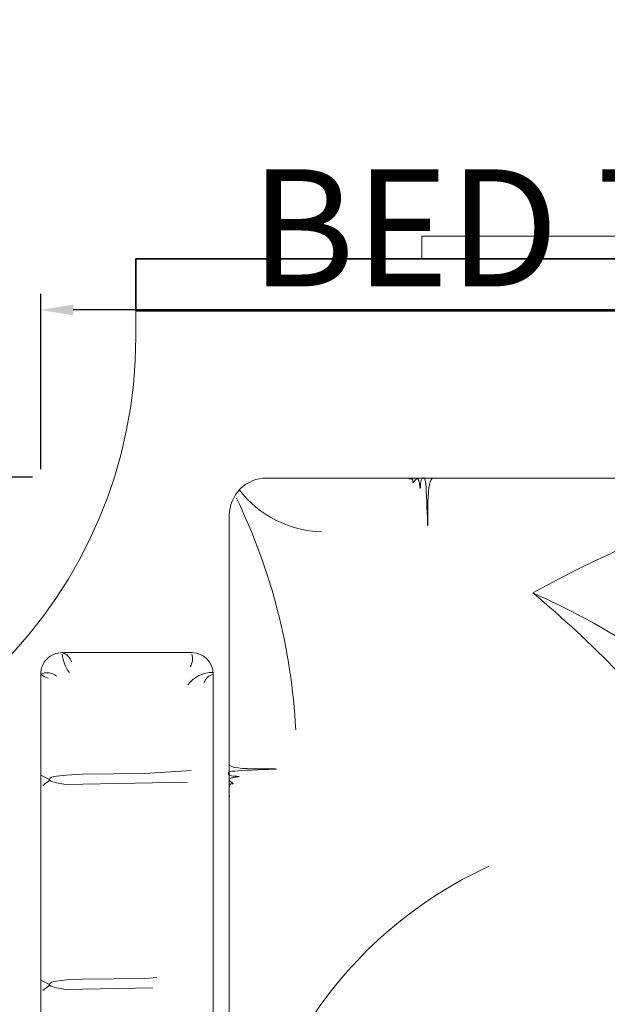
# Model space of a CAD drawing. Units: inches. Extents: x 3321 to 5237, y 11 to 1752.
# Tile 17 of 43: x 4367 to 4413, y 1230 to 1306. Entities that reach past the tile are written whole.
import ezdxf

# ---------------------------------------------------------------- set-up
doc = ezdxf.new("R2010")
doc.units = ezdxf.units.IN
for name, color, linetype, lineweight in [('A-ANNO-DIMS', 2, 'Continuous', 18), ('A-DOOR', 4, 'Continuous', 18), ('A-WALL', 7, 'Continuous', 35), ('FUR', 42, 'Continuous', 18)]:
    doc.layers.add(name, color=color, linetype=linetype, lineweight=lineweight)
doc.styles.get("Standard").update_dxf_attribs({"font": 'arial.ttf'})
doc.dimstyles.new('ISO-25', dxfattribs={"dimtxt": 9, "dimasz": 2.5, "dimexe": 1.25, "dimexo": 0.625, "dimtad": 1, "dimdec": 1, "dimlunit": 3, "dimtxsty": 'Standard', "dimcen": 2.5, "dimclrd": 4, "dimclre": 4, "dimclrt": 256, "dimadec": 0, "dimazin": 0, "dimtfac": 1, "dimtdec": 1, "dimtmove": 0, "dimatfit": 3, "dimfxl": 1, "dimarcsym": 0})

# ---------------------------------------------------------------- blocks, each defined once
blk = doc.blocks.new('*U9')
for p, q in [((-36, 0), (-36, 6)), ((0, 0), (0, 6))]:
    blk.add_line(p, q)
blk.add_lwpolyline([(0, 0), (0, -36), (-1.75, -36), (-1.75, 0)], close=True)
blk.add_arc((0, 0), 36, 180, 270)
blk = doc.blocks.new('*U5')
for p, q in [((0, 0), (0, -6)), ((-30, 0), (-30, -6))]:
    blk.add_line(p, q)
blk.add_lwpolyline([(0, 0), (0, 30), (-1.75, 30), (-1.75, 0)], close=True)
blk.add_arc((0, 0), 30, 90, 180)
blk = doc.blocks.new('*X127')
at = {"color": 0}
for p, q in [((3155.9, 8182.9), (3155.9, 8182.9)), ((3147.8, 8143.4), (3147.8, 8143.4)), ((3283, 8049.6), (3283, 8049.6)), ((3209.5, 8023.9), (3209.5, 8023.9)), ((3251.6, 7997), (3251.6, 7997)), ((3154.1, 7950.7), (3154.1, 7950.7))]:
    blk.add_line(p, q, dxfattribs=at)
blk = doc.blocks.new('*X126')
at = {"color": 0}
for p, q in [((3155.9, 8182.9), (3155.9, 8182.9)), ((3139.8, 7939.7), (3139.8, 7939.7))]:
    blk.add_line(p, q, dxfattribs=at)
blk = doc.blocks.new('*X125')
at = {"color": 0}
for p, q in [((3155.9, 8182.9), (3155.9, 8182.9)), ((3139.8, 7939.7), (3139.8, 7939.7))]:
    blk.add_line(p, q, dxfattribs=at)
blk = doc.blocks.new('*X124')
at = {"color": 0}
for p, q in [((3163, 7776.2), (3163, 7776.2)), ((3422.2, 7761.3), (3422.2, 7761.3)), ((3244.3, 7698.6), (3244.3, 7698.6)), ((3236.2, 7675.7), (3236.2, 7675.7)), ((3340.3, 7689.4), (3340.3, 7689.4))]:
    blk.add_line(p, q, dxfattribs=at)
blk = doc.blocks.new('BED1')
for p, q in [((0, -1000), (0, 800)), ((150, 800), (0, 800)), ((150, 800), (150, -1000)), ((2058.7, 800), (150, 800)), ((528, 800), (528, -1000)), ((211.8, 614.9), (277.5, 585.4)), ((2537.2, 404.9), (2237.2, 404.9)), ((2187.2, 354.9), (2187.2, -545.1)), ((2587.2, -545.1), (2587.2, 354.9)), ((2582, 188.1), (2565.4, 174.8)), ((2566.3, 178.5), (2565.2, 177.4)), ((2565.4, 174.8), (2585.7, 165.4)), ((2566.3, -296.8), (2565.2, -297.9)), ((2582, -287.1), (2565.4, -300.5)), ((2565.4, -300.5), (2585.7, -309.9)), ((2237.2, -595.1), (2537.2, -595.1)), ((150, -1000), (0, -1000)), ((150, -1000), (2063.5, -1000))]:
    blk.add_line(p, q)
for points in [[(934, 797.9), (930.9, 797.7), (928.3, 797.4), (926.3, 796.9), (924.9, 796.3), (923.8, 795.6), (923.1, 794.8), (922.7, 793.8), (922.5, 792.7), (922.4, 791.5), (922.5, 790.3), (922.6, 789.2), (922.6, 788.3), (922.6, 787.6), (922.4, 787.3), (922, 787.4), (921.4, 787.9), (920.6, 788.9), (919.5, 790.2), (918.4, 791.6), (917.1, 793.1), (915.9, 794.6), (914.6, 796), (913.3, 797.1), (912.2, 797.9), (911.1, 798.3), (910.1, 798.4), (909.2, 798), (908.3, 797.1), (907.5, 795.8), (906.8, 793.9), (906, 791.4), (905.4, 788.5), (904.8, 785.2), (904.2, 781.7), (903.7, 778.4), (903.2, 775.4), (902.8, 772.9), (902.5, 771.3), (902.3, 770.6), (902.1, 771.2), (902, 772.8), (901.8, 775.2), (901.7, 778.1), (901.5, 781.5), (901.2, 785), (900.8, 788.4), (900.2, 791.5), (899.5, 794.1), (898.6, 796.2), (897.6, 797.9), (896.5, 799.2), (895.3, 800), (894.1, 800.5), (893, 800.7), (891.9, 800.5), (890.9, 800.1), (890, 799), (889.1, 797.1), (888.3, 794), (887.6, 789.3), (886.9, 782.9), (886.2, 774.2), (885.5, 763.1), (884.8, 749.5), (884.2, 734.2), (883.6, 718.3), (883, 702.8), (882.5, 688.8), (882, 677.5), (881.7, 669.8), (881.5, 666.9), (881.3, 669.4), (881.3, 676.7), (881.3, 687.8), (881.2, 701.5), (881.1, 716.8), (880.8, 732.6), (880.2, 748), (879.4, 761.8), (878.3, 773.2), (876.9, 782.2), (875.1, 789.2), (872.9, 794.4), (870.3, 798), (869, 799)], [(2150, -913.5), (2150, 723.2)], [(2327.6, 182.3), (2530, 185.9), (2550.8, 181.9), (2561.7, 179), (2566, 176.7), (2566.9, 174.4), (2566.3, 171.9), (2562, 169.2), (2550.3, 166.5), (2527.7, 163.9), (2490.6, 161.8), (2345.5, 160.2), (2317.8, 158.5)], [(494.7, 3.1), (458.9, 95.3)], [(2149.7, -259.9), (2150, -268.4), (2150.1, -274.1), (2150.1, -278.1), (2150, -281.4), (2149.8, -284), (2149.5, -286.1), (2149.1, -287.8), (2148.7, -289), (2148.1, -289.9), (2147.4, -290.5), (2146.6, -290.8), (2145.6, -291), (2144.6, -291), (2143.6, -291), (2142.7, -290.9), (2141.9, -290.9), (2141.4, -290.9), (2141.1, -291), (2141.2, -291.4), (2141.7, -291.9), (2142.5, -292.6), (2143.5, -293.4), (2144.7, -294.4), (2146, -295.4), (2147.2, -296.5), (2148.4, -297.6), (2149.3, -298.6), (2150, -299.6), (2150.3, -300.5), (2150.4, -301.3), (2150, -302.1), (2149.3, -302.8), (2148.2, -303.5), (2146.6, -304.1), (2144.6, -304.7), (2142.1, -305.2), (2139.3, -305.7), (2136.5, -306.2), (2133.7, -306.6), (2131.2, -307), (2129.2, -307.3), (2127.8, -307.6), (2127.3, -307.8), (2127.7, -308), (2129, -308.1), (2131, -308.2), (2133.5, -308.3), (2136.3, -308.5), (2139.2, -308.7), (2142, -309), (2144.6, -309.5), (2146.8, -310.1), (2148.6, -310.9), (2150, -311.7), (2151, -312.7), (2151.7, -313.6), (2152.1, -314.6), (2152.3, -315.6), (2152.2, -316.5), (2151.8, -317.3), (2150.9, -318.1), (2149.3, -318.8), (2146.7, -319.4), (2142.8, -320), (2137.4, -320.6), (2130.2, -321.2), (2121, -321.8), (2109.7, -322.3), (2096.9, -322.9), (2083.6, -323.4), (2070.7, -323.9), (2059.1, -324.3), (2049.6, -324.7), (2043.2, -325), (2040.8, -325.2), (2042.9, -325.3), (2049, -325.3), (2058.2, -325.3), (2069.6, -325.4), (2082.3, -325.5), (2095.6, -325.8), (2108.4, -326.2), (2119.9, -326.8), (2129.4, -327.8), (2136.9, -329), (2142.7, -330.5), (2147, -332.3), (2150, -334.4), (2150.9, -335.6)], [(2246.5, -294.4), (2530, -289.4), (2550.8, -293.4), (2561.7, -296.3), (2566, -298.6), (2566.9, -300.8), (2566.3, -303.4), (2562, -306.1), (2550.3, -308.8), (2527.7, -311.3), (2490.6, -313.5), (2345.5, -315), (2238.6, -321.8)], [(1733.7, -998.3), (1731.1, -998.1), (1729, -997.8), (1727.4, -997.4), (1726.1, -997), (1725.2, -996.4), (1724.7, -995.7), (1724.3, -994.8), (1724.1, -993.9), (1724.1, -992.9), (1724.1, -991.9), (1724.2, -991), (1724.2, -990.2), (1724.2, -989.7), (1724.1, -989.4), (1723.8, -989.5), (1723.2, -990), (1722.5, -990.8), (1721.7, -991.8), (1720.7, -993), (1719.7, -994.3), (1718.6, -995.5), (1717.5, -996.6), (1716.5, -997.6), (1715.5, -998.3), (1714.6, -998.6), (1713.8, -998.6), (1713, -998.3), (1712.3, -997.6), (1711.7, -996.5), (1711, -994.9), (1710.4, -992.9), (1709.9, -990.4), (1709.4, -987.6), (1708.9, -984.8), (1708.5, -982), (1708.1, -979.5), (1707.8, -977.4), (1707.5, -976.1), (1707.3, -975.5), (1707.1, -976), (1707, -977.3), (1706.9, -979.3), (1706.8, -981.8), (1706.7, -984.6), (1706.4, -987.5), (1706.1, -990.3), (1705.6, -992.9), (1705, -995.1), (1704.2, -996.9), (1703.4, -998.3), (1702.4, -999.3), (1701.5, -1000), (1700.5, -1000.4), (1699.6, -1000.6), (1698.7, -1000.4), (1697.8, -1000.1), (1697, -999.2), (1696.3, -997.6), (1695.7, -995), (1695.1, -991.1), (1694.5, -985.7), (1693.9, -978.5), (1693.3, -969.3), (1692.8, -957.9), (1692.2, -945.2), (1691.7, -931.9), (1691.2, -919), (1690.8, -907.4), (1690.4, -897.9), (1690.1, -891.5), (1689.9, -889.1), (1689.8, -891.2), (1689.8, -897.3), (1689.8, -906.5), (1689.7, -917.9), (1689.6, -930.6), (1689.4, -943.8), (1688.9, -956.6), (1688.3, -968.1), (1687.3, -977.6), (1686.1, -985.2), (1684.6, -991), (1682.8, -995.3), (1680.7, -998.3), (1679.6, -999.2)]]:
    blk.add_lwpolyline(points)
for points in [[(205.5, 619.6, 0.267769), (215.1, 582.4, -0.037739), (204.3, 21.8, 0.684696), (236.7, 5.5, -0.060702), (497.2, 0.1, -0.046649), (225.9, 3.1, -1.318436)], [(489.2, 619.6, 0.144019), (207.6, 617.9, 0.248643)], [(497.2, 0.1, 0.021276), (489.2, 619.6, -0.206383), (326.6, 509.4, 0.237198)], [(211.8, 12.8, 0.143972), (361.6, 262.9, 1.292232)], [(886.4, -150, -0.069098), (985, -66.5, 0.658965), (982.1, -48.7, -0.049789), (927.4, -29, -0.103757), (896.6, -5.4, 0.055725), (800.9, 83.3, -0.11866), (782.7, 104.9, 0.016811), (761.6, 143.9, 0.70791), (748.3, 144, -0.16964), (551.9, -96.6, 0.664036), (554, -110.7, 0.023706), (627, -144.7, -0.134834), (683.2, -188, 0.012748), (746.3, -267.4)], [(969.1, -259.1, 0.263265), (936.3, -236.9, -0.026108), (909.2, -233.2, 0.027613), (945.1, -234.2, -0.089259), (872.7, -120, 0.662242), (857.6, -119.3, -0.162037), (651.8, -332.7, 0.676499), (654, -354.5, -0.160513), (722.9, -401.5, 0.07473), (773.5, -450.3, -0.187721), (845.5, -559.9, 0.70791), (858.8, -561.4, -0.010003), (898.6, -497.3, -0.113819), (947.3, -450.2, 0.099539), (1032.5, -372.4, -0.173425), (1070.9, -346.4, 0.589988), (1076.2, -326.1, 0.137312), (923.9, -245.9, 0.137312)], [(489.2, -168.2, 0.144019), (207.6, -169.9, 0.248643)], [(205.5, -168.2, 0.267769), (215.1, -205.4, -0.037739), (204.3, -766, 0.684696), (236.7, -782.3, -0.060702), (497.2, -787.7, -0.046649), (225.9, -784.7, -1.318436)], [(497.2, -787.7, 0.021276), (489.2, -168.2, -0.206383), (326.6, -278.4, 0.237198)], [(1446, -733.4, -0.095039), (652.8, -1001.7)]]:
    blk.add_lwpolyline(points, format="xyb")
for centre, radius, start, end in [((3208.8, 1363.3), 2739.4, 191.8679, 206.3247), ((2062.7, 713.7), 86.5, 0, 93.5376), ((1608.1, 842.5), 496.3, 305.1901, 354.0206), ((1138.6, 793.9), 983.2, 294.6078, 358.3033), ((2237.2, 354.9), 50, 90, 180), ((2321.1, 409.7), 84.5, 185.6196, 217.1396), ((2227.5, 373.5), 32.8, 17.833, 72.8005), ((2546.9, 373.5), 32.8, 107.1995, 162.167), ((2453.3, 409.7), 84.5, 322.8604, 354.3804), ((2537.2, 354.9), 50, 0, 90), ((2098.7, 754.7), 1625, 193.905, 207.8169), ((2201.9, 323.3), 34.8, 50.8413, 114.9586), ((2212.2, 381.5), 36.5, 226.8095, 258.3841), ((2572.5, 323.3), 34.8, 65.0414, 129.1587), ((2562.2, 381.5), 36.5, 281.6159, 313.1905), ((751.8, 88.7), 34.9, 336.8352, 27.7218), ((684.2, 86), 100.3, 353.675, 10.882), ((1074.1, 198.8), 306.1, 197.8602, 241.5122), ((341.4, -277.7), 318.5, 60.7125, 115.009), ((983.7, -79.5), 20.8, 73.7967, 130.4566), ((978.5, -68.6), 14.3, 39.7097, 85.9506), ((602.5, -324), 198.6, 43.2035, 95.0556), ((3208.8, 1363.3), 2739.4, 212.9314, 216.951), ((981.1, -281.8), 131.1, 164.0372, 243.4536), ((980, -379), 163.4, 152.6104, 209.361), ((3208.8, 1363.3), 2739.4, 218.6329, 229.9449), ((2098.7, 754.7), 1625, 226.5887, 246.3156), ((3402.5, -342.9), 1408.5, 182.9917, 205.6819), ((2188.1, -476.2), 73, 269.4513, 322.8027), ((-34.4, -471.2), 376.5, 312.0118, 350.9635), ((2178, -513.5), 33, 286.1827, 338.1386), ((2237.2, -545.1), 50, 180, 270), ((2537.2, -545.1), 50, 270, 0), ((2572.5, -513.6), 34.8, 230.8413, 294.9586), ((2562.2, -571.8), 36.5, 46.8095, 78.3841), ((2271.1, -580.9), 35.8, 148.9055, 197.5541), ((2453.3, -600), 84.5, 5.6196, 37.1396), ((2546.9, -563.8), 32.8, 197.833, 252.8005), ((375.7, -807.4), 128.2, 17.4073, 88.5129), ((341.4, -1065.5), 318.5, 60.7125, 115.009), ((1929.1, -1126), 250.5, 37.8553, 88.4405), ((2063.5, -913.5), 86.5, 270, 0)]:
    blk.add_arc(centre, radius, start, end)
for name in ['*X126', '*X125', '*X127', '*X124']:
    blk.add_blockref(name, (-2425.3, -8101.4))
blk = doc.blocks.new('*D195')
at = {"layer": 'A-ANNO-DIMS', "color": 4, "lineweight": -2, "transparency": 16777216}
for p, q in [((4369.073, 1271.165), (4369.073, 1284.663)), ((4454.896, 1271.165), (4454.896, 1284.663)), ((4452.396, 1283.413), (4371.573, 1283.413))]:
    blk.add_line(p, q, dxfattribs=at)
at = {"layer": 'A-ANNO-DIMS', "color": 4, "transparency": 16777216}
for points in [[(4371.573, 1283.83), (4371.573, 1282.997), (4369.073, 1283.413)], [(4452.396, 1283.83), (4452.396, 1282.997), (4454.896, 1283.413)]]:
    blk.add_solid(points, dxfattribs=at)
at = {"layer": 'Defpoints', "color": 0, "transparency": 16777216}
for p in [(4369.073, 1283.413), (4369.073, 1270.54), (4454.896, 1270.54)]:
    blk.add_point(p, dxfattribs=at)
at = {"layer": 'A-ANNO-DIMS', "transparency": 16777216, "insert": (4411.984, 1288.56), "char_height": 9, "attachment_point": 5}
blk.add_mtext('BED 7\'-2"', dxfattribs=at)
blk = doc.blocks.new('*D196')
at = {"layer": 'A-ANNO-DIMS', "color": 4, "lineweight": -2, "transparency": 16777216}
for p, q in [((4368.448, 1270.54), (4354.95, 1270.54)), ((4356.2, 1268.04), (4356.2, 1213.226)), ((4368.448, 1210.726), (4354.95, 1210.726))]:
    blk.add_line(p, q, dxfattribs=at)
at = {"layer": 'A-ANNO-DIMS', "color": 4, "transparency": 16777216}
for points in [[(4355.783, 1268.04), (4356.616, 1268.04), (4356.2, 1270.54)], [(4355.783, 1213.226), (4356.616, 1213.226), (4356.2, 1210.726)]]:
    blk.add_solid(points, dxfattribs=at)
at = {"layer": 'Defpoints', "color": 0, "transparency": 16777216}
for p in [(4369.073, 1270.54), (4356.2, 1210.726), (4369.073, 1210.726)]:
    blk.add_point(p, dxfattribs=at)
at = {"layer": 'A-ANNO-DIMS', "transparency": 16777216, "insert": (4350.98, 1240.633), "char_height": 9, "attachment_point": 5, "rotation": 90}
blk.add_mtext('5\'-0"', dxfattribs=at)

msp = doc.modelspace()

# ---------------------------------------------------------------- linework, layer by layer
at = {"layer": 'A-WALL'}
for p, q in [((4376.386, 1287.339), (4376.386, 1283.339)), ((4376.386, 1287.339), (4456.386, 1287.339)), ((4376.386, 1283.339), (4456.386, 1283.339))]:
    msp.add_line(p, q, dxfattribs=at)

# ---------------------------------------------------------------- block references
at = {"layer": 'A-DOOR', "rotation": 270}
msp.add_blockref('*U5', (4398.386, 1287.339), dxfattribs=at)
at = {"layer": 'A-DOOR', "xscale": -1}
msp.add_blockref('*U9', (4340.386, 1281.339), dxfattribs=at)
at = {"layer": 'FUR', "xscale": 0.0331718847221821, "yscale": 0.0331718847221821, "zscale": 0.0331718847221821, "rotation": 180}
msp.add_blockref('BED1', (4454.896, 1237.313), dxfattribs=at)

# ---------------------------------------------------------------- dimensions: what is measured, and where the dimension line sits
at = {"layer": 'A-ANNO-DIMS'}
dim = msp.add_linear_dim(base=(4369.073, 1283.413), p1=(4454.896, 1270.54), p2=(4369.073, 1270.54), angle=180, text='BED <>', dimstyle='ISO-25', override={"dimdec": 1, "dimlfac": 1, "dimrnd": 0, "dimzin": 1, "dimdsep": 46, "dimlunit": 4, "dimfrac": 2}, dxfattribs=at)
dim.commit()
dim.dimension.update_dxf_attribs({"geometry": '*D195', "text_midpoint": (4411.984, 1288.56)})
dim = msp.add_linear_dim(base=(4356.2, 1210.726), p1=(4369.073, 1270.54), p2=(4369.073, 1210.726), angle=270, dimstyle='ISO-25', override={"dimdec": 1, "dimlfac": 1, "dimrnd": 0, "dimzin": 1, "dimdsep": 46, "dimlunit": 4, "dimfrac": 2}, dxfattribs=at)
dim.commit()
dim.dimension.update_dxf_attribs({"geometry": '*D196', "text_midpoint": (4350.98, 1240.633)})

doc.saveas('drawing.dxf')
